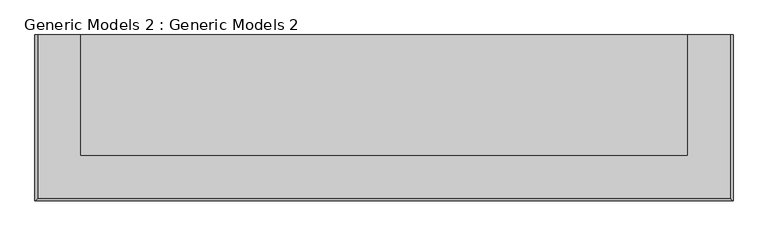
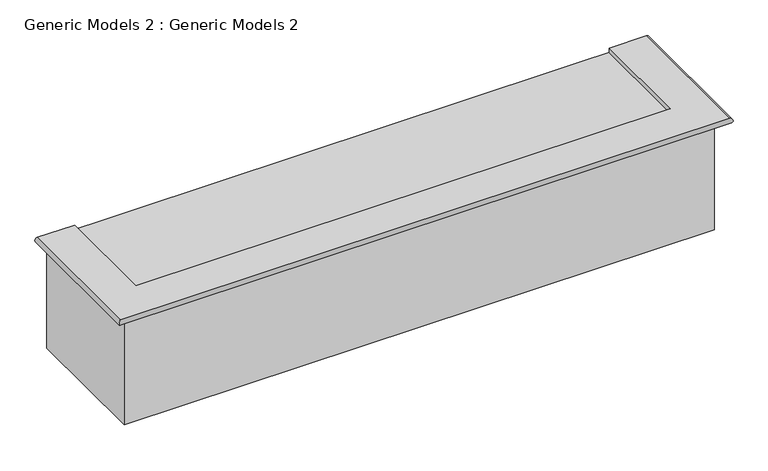
"""IFC4 building model written with IfcOpenShell, lengths in millimetres: proxy geometry, Generic Models 2 : Generic Models 2."""

from ifc_helpers import new_model, si_unit, frame, origin, origin_with_axes, place, context, project, spatial, polyline, circle_curve, ellipse_curve, outline, extrude, source, transform, mapped, element, save
from ifc_brep_helpers import plane_surface, cylinder_surface, advanced_brep


def generic_models_2_generic_models_2_8e2cd793(model_context):
    return source(origin(), model_context, "Body", "SolidModel", [
        advanced_brep(
        [(3296.7271331, -11975.7643494, 609.6), (3296.7271331, -11975.7643494, 635.0), (3493.9217895, -11975.7643494, 635.0), (3493.9217895, -11975.7643494, 609.6), (3296.7271331, -12732.6919489, 609.6), (3296.7271331, -12732.6919489, 635.0), (6508.5191987, -12732.6919489, 635.0), (6508.5191987, -11975.7643494, 635.0), (6311.3245424, -11975.7643494, 635.0), (6311.3245424, -12535.4972925, 635.0), (3493.9217895, -12535.4972925, 635.0), (3493.9217895, -12535.4972925, 609.6), (6311.3245424, -12535.4972925, 609.6), (6311.3245424, -11975.7643494, 609.6), (6508.5191987, -11975.7643494, 609.6), (6508.5191987, -12732.6919489, 609.6)],
        [
            (0, 1, circle_curve(frame((3296.7271331, -11975.7643494, 622.3), z_axis=(0.0, 1.0, 0.0), x_axis=(1.0, 0.0, 0.0)), 12.7)),
            (1, 2),
            (2, 3),
            (3, 0),
            (0, 4),
            (4, 5, ellipse_curve(frame((3296.7271331, -12732.6919489, 622.3), z_axis=(-0.7071067811865475, 0.7071067811865475, 0.0), x_axis=(0.7071067811865474, 0.7071067811865476, 0.0)), 17.9605122, 12.7)),
            (5, 1),
            (5, 6),
            (6, 7),
            (7, 8),
            (8, 9),
            (9, 10),
            (10, 2),
            (10, 11),
            (11, 3),
            (11, 12),
            (12, 13),
            (13, 14),
            (14, 15),
            (15, 4),
            (15, 6, ellipse_curve(frame((6508.5191987, -12732.6919489, 622.3), z_axis=(-0.7071067811865475, -0.7071067811865475, 0.0), x_axis=(-0.7071067811865476, 0.7071067811865474, 0.0)), 17.9605122, 12.7)),
            (9, 12),
            (13, 8),
            (7, 14, circle_curve(frame((6508.5191987, -11975.7643494, 622.3), z_axis=(0.0, 1.0, 0.0), x_axis=(-1.0, 0.0, 0.0)), 12.7)),
        ],
        [
            plane_surface(frame((3347.5271331, -11975.7643494, 609.6), z_axis=(0.0, 1.0, 0.0), x_axis=(0.0, 0.0, 1.0))),
            cylinder_surface(frame((3296.7271331, -11975.7643494, 622.3), z_axis=(0.0, 1.0, 0.0), x_axis=(1.0, 0.0, 0.0)), 12.7),
            plane_surface(frame((3296.7271331, -11975.7643494, 635.0), z_axis=(0.0, 0.0, 1.0), x_axis=(0.0, -1.0, 0.0))),
            plane_surface(frame((3493.9217895, -11975.7643494, 635.0), z_axis=(1.0, 0.0, 0.0), x_axis=(0.0, -1.0, 0.0))),
            plane_surface(frame((3493.9217895, -11975.7643494, 609.6), z_axis=(0.0, 0.0, -1.0), x_axis=(0.0, -1.0, 0.0))),
            cylinder_surface(frame((3347.5271331, -12732.6919489, 622.3), z_axis=(-1.0, 0.0, 0.0), x_axis=(0.0, 1.0, 0.0)), 12.7),
            plane_surface(frame((3493.9217895, -12535.4972925, 635.0), z_axis=(0.0, 1.0, 0.0), x_axis=(1.0, 0.0, 0.0))),
            plane_surface(frame((6457.7191987, -11975.7643494, 609.6), z_axis=(0.0, 1.0, 0.0), x_axis=(0.0, 0.0, 1.0))),
            cylinder_surface(frame((6508.5191987, -12681.8919489, 622.3), z_axis=(0.0, -1.0, 0.0), x_axis=(-1.0, 0.0, 0.0)), 12.7),
            plane_surface(frame((6311.3245424, -12535.4972925, 635.0), z_axis=(-1.0, 0.0, 0.0), x_axis=(0.0, 1.0, 0.0))),
        ],
        [
            (0, [[1, 2, 3, 4]]),
            (1, [[-1, 5, 6, 7]]),
            (2, [[-2, -7, 8, 9, 10, 11, 12, 13]]),
            (3, [[-3, -13, 14, 15]]),
            (4, [[-4, -15, 16, 17, 18, 19, 20, -5]]),
            (5, [[-6, -20, 21, -8]]),
            (6, [[-14, -12, 22, -16]]),
            (7, [[-18, 23, -10, 24]]),
            (8, [[-21, -19, -24, -9]]),
            (9, [[-22, -11, -23, -17]]),
        ],
    ),
        extrude(outline(polyline([(6457.7191987, -11975.7643494), (6457.7191987, -12681.8919489), (3347.5271331, -12681.8919489), (3347.5271331, -11975.7643494), (6457.7191987, -11975.7643494)])), origin_with_axes(), (0.0, 0.0, 1.0), 609.6),
    ])


if __name__ == "__main__":
    model = new_model("IFC4")
    model_context = context("Model", 3, world=origin())
    ifc_project = project(units=[si_unit("LENGTHUNIT", "METRE", prefix="MILLI")], contexts=[model_context])
    site = spatial("IfcSite", under=ifc_project)
    building = spatial("IfcBuilding", under=site)
    placement = place(None, origin())
    generic_models_2_generic_models_2_shape = generic_models_2_generic_models_2_8e2cd793(model_context)
    element("IfcBuildingElementProxy", 1, Name="Generic Models 2 : Generic Models 2", ObjectType="Generic Models 2 : Generic Models 2", at=placement, inside=building, context=model_context, shape_type="MappedRepresentation", body=[
        mapped(generic_models_2_generic_models_2_shape, transform((0.0, 0.0, 0.0), x_axis=(1.0, 0.0, 0.0), y_axis=(0.0, 1.0, 0.0), z_axis=(0.0, 0.0, 1.0))),
    ])
    save(model, "model.ifc")

# Revit data of these elements
# Element 1 (IfcBuildingElementProxy, "Generic Models 2 : Generic Models 2")
#   Materials on its faces: "Roofing, EPDM Membrane", "Oak Flooring", "Tile, Mosaic, Gray"
# Materials
#   "Roofing, EPDM Membrane": class "Generic", colour RGB 127 127 127, transparency 0, Description = "EPDM roof membrane", Cost = 0
#   "Oak Flooring": class "Wood", colour RGB 216 169 114, transparency 0, Description = "Quercus Rubra", Cost = 0
#   "Tile, Mosaic, Gray": class "Generic", colour RGB 127 127 127, transparency 0, Description = "Mosiac tile, gray", Cost = 0
